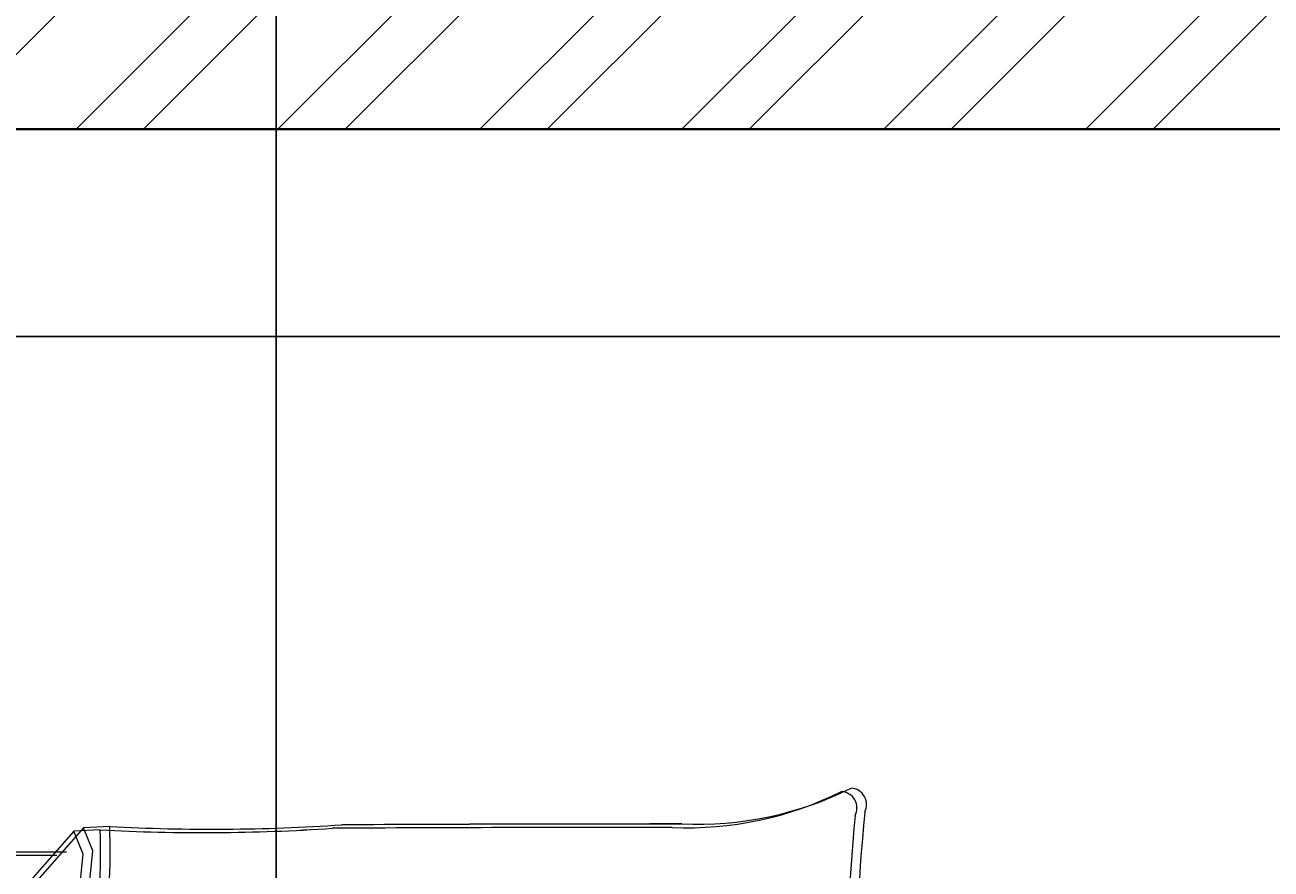
# Model space of a CAD drawing. Units: inches. Extents: x 1601 to 2297, y 1496 to 2631.
# Tile 12 of 57: x 1723 to 1806, y 1973 to 2029. Entities that reach past the tile are written whole.
import ezdxf

# ---------------------------------------------------------------- set-up
doc = ezdxf.new("R2010")
doc.units = ezdxf.units.IN
for name, color, linetype, lineweight in [('A-ANNO-DIMS', 2, 'Continuous', 18), ('A-FURN', 8, 'Continuous', 18), ('A-WALL', 7, 'Continuous', 40), ('A-WALL-PATT', 215, 'Continuous', 13)]:
    doc.layers.add(name, color=color, linetype=linetype, lineweight=lineweight)
doc.styles.get("Standard").update_dxf_attribs({"font": 'arial.ttf'})
doc.dimstyles.get("Standard").update_dxf_attribs({"dimtxt": 0.18, "dimasz": 0.18, "dimexe": 0.18, "dimexo": 0.0625, "dimgap": 0.09, "dimtad": 0, "dimtih": 1, "dimtoh": 1, "dimdec": 4, "dimzin": 0, "dimdsep": 46, "dimtxsty": 'Standard', "dimcen": 0.09, "dimadec": 0, "dimazin": 0, "dimtfac": 1, "dimtdec": 4, "dimtofl": 0, "dimtmove": 0, "dimatfit": 3, "dimfxl": 1, "dimtolj": 1, "dimtzin": 0, "dimarcsym": 0})

# ---------------------------------------------------------------- blocks, each defined once
blk = doc.blocks.new('BED-DOUBLE')
for p, q in [((27.746, 52.867), (24.495, 49.162)), ((27.746, 52.867), (24.495, 49.162)), ((27.746, 52.867), (24.495, 49.162)), ((27.746, 52.867), (24.495, 49.162)), ((28.385, 53.096), (25.135, 49.39)), ((28.385, 53.096), (25.135, 49.39)), ((28.385, 53.096), (25.135, 49.39)), ((28.385, 53.096), (25.135, 49.39)), ((29.49, 52.947), (27.746, 52.867, 3.871)), ((29.49, 52.947), (27.746, 52.867, 3.871)), ((29.49, 52.947), (27.746, 52.867, 3.871)), ((29.49, 52.947), (27.746, 52.867, 3.871)), ((28.365, 51.33), (27.746, 52.867)), ((28.365, 51.33), (27.746, 52.867)), ((28.365, 51.33), (27.746, 52.867)), ((28.365, 51.33), (27.746, 52.867)), ((30.13, 53.175), (28.385, 53.096, 3.871)), ((30.13, 53.175), (28.385, 53.096, 3.871)), ((30.13, 53.175), (28.385, 53.096, 3.871)), ((30.13, 53.175), (28.385, 53.096, 3.871)), ((29.004, 51.559), (28.385, 53.096)), ((29.004, 51.558), (28.385, 53.096)), ((29.004, 51.559), (28.385, 53.096)), ((29.004, 51.558), (28.385, 53.096)), ((28.695, 48.461), (29.004, 51.559)), ((28.695, 48.461), (29.004, 51.559)), ((28.695, 48.461), (29.004, 51.558)), ((28.695, 48.461), (29.004, 51.558)), ((0, 51.494), (0.639, 51.493)), ((0, 3.475), (0, 51.494)), ((0, 51.494), (0.639, 51.493)), ((0, 3.475), (0, 51.494)), ((0, 51.265), (26.61, 51.265)), ((0, 51.265), (26.61, 51.265)), ((0, 51.265), (26.61, 51.265)), ((0, 51.265), (26.61, 51.265)), ((0.639, 51.494), (27.249, 51.494)), ((0.639, 51.494), (27.249, 51.494)), ((0.639, 51.493), (27.249, 51.493)), ((0.639, 51.493), (27.249, 51.493)), ((1.533, 3.475), (1.533, 51.265)), ((1.533, 3.475), (1.533, 51.265)), ((1.533, 3.475), (1.533, 51.265)), ((1.533, 3.475), (1.533, 51.265)), ((2.173, 3.703), (2.173, 51.494)), ((2.173, 3.703), (2.173, 51.494)), ((2.173, 3.703), (2.173, 51.493)), ((2.173, 3.703), (2.173, 51.493)), ((17.212, 50.926), (14.073, 50.151)), ((17.212, 50.926), (14.073, 50.151)), ((17.212, 50.926), (14.073, 50.151)), ((17.212, 50.926), (14.073, 50.151)), ((16.808, 45.795), (17.212, 50.926)), ((16.808, 45.794), (17.212, 50.926)), ((16.808, 45.795), (17.212, 50.926)), ((16.808, 45.794), (17.212, 50.926)), ((28.055, 48.233), (28.365, 51.33)), ((28.055, 48.233), (28.365, 51.33)), ((28.055, 48.233), (28.365, 51.33)), ((28.055, 48.233), (28.365, 51.33)), ((2.557, 50.112), (2.46, 44.709)), ((2.557, 50.112), (2.46, 44.709)), ((2.557, 50.111), (2.46, 44.709)), ((2.557, 50.111), (2.46, 44.709)), ((2.557, 50.112), (5.768, 49.733)), ((2.557, 50.112), (5.768, 49.733)), ((2.557, 50.111), (5.768, 49.733)), ((2.557, 50.111), (5.768, 49.733)), ((3.196, 50.34), (3.099, 44.938)), ((3.196, 50.34), (3.099, 44.938)), ((3.196, 50.34), (3.099, 44.938)), ((3.196, 50.34), (3.099, 44.938)), ((3.196, 50.34), (6.407, 49.961)), ((3.196, 50.34), (6.407, 49.961)), ((3.196, 50.34), (6.407, 49.961)), ((3.196, 50.34), (6.407, 49.961)), ((5.768, 49.733), (8.338, 50.328)), ((5.768, 49.733), (8.338, 50.328)), ((5.768, 49.733), (8.338, 50.328)), ((5.768, 49.733), (8.338, 50.328)), ((6.407, 49.961), (8.977, 50.557)), ((6.407, 49.961), (8.977, 50.557)), ((6.407, 49.961), (8.977, 50.556)), ((6.407, 49.961), (8.977, 50.556)), ((11.829, 50.112), (8.257, 49.309)), ((11.829, 50.112), (8.257, 49.309)), ((11.829, 50.112), (8.257, 49.309)), ((11.829, 50.112), (8.257, 49.309)), ((8.338, 50.328), (9.384, 49.814)), ((8.338, 50.328), (9.384, 49.814)), ((8.338, 50.328), (9.384, 49.814)), ((8.338, 50.328), (9.384, 49.814)), ((12.468, 50.34), (8.896, 49.538)), ((12.468, 50.34), (8.896, 49.537)), ((12.468, 50.34), (8.896, 49.538)), ((12.468, 50.34), (8.896, 49.537)), ((8.977, 50.557), (10.024, 50.043)), ((8.977, 50.557), (10.024, 50.043)), ((8.977, 50.556), (10.024, 50.042)), ((8.977, 50.556), (10.024, 50.042)), ((13.434, 49.923), (11.829, 50.112)), ((13.434, 49.922), (11.829, 50.112)), ((13.434, 49.923), (11.829, 50.112)), ((13.434, 49.922), (11.829, 50.112)), ((14.073, 50.151), (12.468, 50.34)), ((14.073, 50.151), (12.468, 50.34)), ((14.073, 50.151), (12.468, 50.34)), ((14.073, 50.151), (12.468, 50.34)), ((16.573, 50.698), (13.434, 49.923)), ((16.573, 50.698), (13.434, 49.922)), ((16.573, 50.698), (13.434, 49.923)), ((16.573, 50.698), (13.434, 49.922)), ((16.169, 45.566), (16.573, 50.698)), ((16.169, 45.566), (16.573, 50.698)), ((16.169, 45.566), (16.573, 50.698)), ((16.169, 45.566), (16.573, 50.698)), ((8.257, 49.309), (5.578, 48.128)), ((8.257, 49.309), (5.578, 48.128)), ((8.257, 49.309), (5.578, 48.128)), ((8.257, 49.309), (5.578, 48.128)), ((8.896, 49.538), (6.218, 48.356)), ((8.896, 49.538), (6.218, 48.356)), ((8.896, 49.537), (6.218, 48.356)), ((8.896, 49.537), (6.218, 48.356)), ((24.495, 49.162), (22.329, 46.219)), ((24.495, 49.162), (22.329, 46.219)), ((24.495, 49.162), (22.329, 46.219)), ((24.495, 49.162), (22.329, 46.219)), ((25.135, 49.39), (22.968, 46.448)), ((25.135, 49.39), (22.968, 46.448)), ((25.135, 49.39), (22.968, 46.448)), ((25.135, 49.39), (22.968, 46.448)), ((28.365, 44.361), (28.055, 48.233)), ((28.365, 44.361), (28.055, 48.233)), ((28.365, 44.361), (28.055, 48.233)), ((28.365, 44.361), (28.055, 48.233)), ((29.004, 44.589), (28.695, 48.461)), ((29.004, 44.589), (28.695, 48.461)), ((29.004, 44.589), (28.695, 48.461)), ((29.004, 44.589), (28.695, 48.461)), ((3.099, 44.938), (3.181, 45.941)), ((3.099, 44.938), (3.181, 45.941)), ((3.099, 44.938), (3.181, 45.94)), ((3.099, 44.938), (3.181, 45.94)), ((3.181, 45.941), (3.709, 42.143)), ((3.181, 45.941), (3.709, 42.143)), ((3.181, 45.94), (3.709, 42.142)), ((3.181, 45.94), (3.709, 42.142)), ((17.365, 43.834), (16.808, 45.795)), ((17.365, 43.834), (16.808, 45.795)), ((17.365, 43.834), (16.808, 45.794)), ((17.365, 43.834), (16.808, 45.794)), ((22.329, 46.219), (20.316, 40.644)), ((22.329, 46.219), (20.316, 40.644)), ((22.329, 46.219), (20.317, 40.644)), ((22.329, 46.219), (20.317, 40.644)), ((22.968, 46.448), (20.956, 40.872)), ((22.968, 46.448), (20.956, 40.872)), ((22.968, 46.448), (20.956, 40.872)), ((22.968, 46.448), (20.956, 40.872)), ((2.46, 44.709), (2.542, 45.712)), ((2.46, 44.709), (2.542, 45.712)), ((2.46, 44.709), (2.542, 45.712)), ((2.46, 44.709), (2.542, 45.712)), ((2.542, 45.712), (3.069, 41.914)), ((2.542, 45.712), (3.069, 41.914)), ((2.542, 45.712), (3.069, 41.914)), ((2.542, 45.712), (3.069, 41.914)), ((16.726, 43.606), (16.169, 45.566)), ((16.726, 43.606), (16.169, 45.566)), ((16.726, 43.606), (16.169, 45.566)), ((16.726, 43.606), (16.169, 45.566)), ((28.829, 40.954), (28.365, 44.361)), ((28.829, 40.953), (28.365, 44.361)), ((28.829, 40.954), (28.365, 44.361)), ((28.829, 40.953), (28.365, 44.361)), ((29.468, 41.182), (29.004, 44.589)), ((29.469, 41.182), (29.004, 44.589)), ((29.468, 41.182), (29.004, 44.589)), ((29.469, 41.182), (29.004, 44.589)), ((16.295, 36.596), (16.726, 43.606)), ((16.295, 36.596), (16.726, 43.606)), ((16.295, 36.596), (16.726, 43.606)), ((16.295, 36.596), (16.726, 43.606)), ((16.934, 36.824), (17.365, 43.834)), ((16.934, 36.824), (17.365, 43.834)), ((16.934, 36.824), (17.365, 43.834)), ((16.934, 36.824), (17.365, 43.834)), ((3.069, 41.914), (4.422, 36.495)), ((3.069, 41.914), (4.422, 36.495)), ((3.069, 41.914), (4.422, 36.495)), ((3.069, 41.914), (4.422, 36.495)), ((3.709, 42.143), (5.061, 36.723)), ((3.709, 42.143), (5.061, 36.723)), ((3.709, 42.142), (5.061, 36.723)), ((3.709, 42.142), (5.061, 36.723)), ((20.956, 40.872), (18.022, 32.534)), ((20.956, 40.872), (18.022, 32.534)), ((20.956, 40.872), (18.022, 32.534)), ((20.956, 40.872), (18.022, 32.534)), ((29.758, 38.94), (28.829, 40.954)), ((29.758, 38.94), (28.829, 40.954)), ((29.758, 38.94), (28.829, 40.953)), ((29.758, 38.94), (28.829, 40.953)), ((30.397, 39.169), (29.468, 41.182)), ((30.397, 39.169), (29.468, 41.182)), ((30.397, 39.168), (29.469, 41.182)), ((30.397, 39.168), (29.469, 41.182)), ((20.316, 40.644), (17.383, 32.306)), ((20.317, 40.644), (17.383, 32.306)), ((20.316, 40.644), (17.383, 32.306)), ((20.317, 40.644), (17.383, 32.306)), ((79.884, 15.292), (79.884, 39.905)), ((79.884, 15.291), (79.884, 39.905)), ((79.884, 15.292), (79.884, 39.905)), ((79.884, 15.291), (79.884, 39.905)), ((3.673, 39.2), (3.078, 37.135)), ((3.673, 39.2), (3.078, 37.135)), ((3.673, 39.2), (3.078, 37.135)), ((3.673, 39.2), (3.078, 37.135)), ((4.313, 39.428), (3.717, 37.363)), ((4.313, 39.428), (3.717, 37.363)), ((4.313, 39.428), (3.718, 37.363)), ((4.313, 39.428), (3.718, 37.363)), ((31.016, 36.691), (30.397, 39.169)), ((31.016, 36.691), (30.397, 39.169)), ((31.016, 36.691), (30.397, 39.168)), ((31.016, 36.691), (30.397, 39.168)), ((79.245, 15.063), (79.245, 39.677)), ((79.245, 15.063), (79.245, 39.677)), ((79.245, 15.063), (79.245, 39.677)), ((79.245, 15.063), (79.245, 39.677)), ((30.377, 36.462), (29.758, 38.94)), ((30.377, 36.462), (29.758, 38.94)), ((30.377, 36.462), (29.758, 38.94)), ((30.377, 36.462), (29.758, 38.94)), ((3.078, 37.135), (2.537, 34.204)), ((3.078, 37.135), (2.537, 34.204)), ((3.078, 37.135), (2.537, 34.204)), ((3.078, 37.135), (2.537, 34.204)), ((3.717, 37.363), (3.176, 34.433)), ((3.718, 37.363), (3.176, 34.433)), ((3.717, 37.363), (3.176, 34.433)), ((3.718, 37.363), (3.176, 34.433)), ((15.628, 32.564), (16.295, 36.596)), ((15.628, 32.564), (16.295, 36.596)), ((15.628, 32.564), (16.295, 36.596)), ((15.628, 32.564), (16.295, 36.596)), ((16.268, 32.792), (16.934, 36.824)), ((16.268, 32.792), (16.934, 36.824)), ((16.268, 32.792), (16.934, 36.824)), ((16.268, 32.792), (16.934, 36.824)), ((29.004, 36.381), (31.016, 36.691)), ((29.004, 36.381), (31.016, 36.691)), ((29.004, 36.381), (31.016, 36.691)), ((29.004, 36.381), (31.016, 36.691)), ((23.876, 34.449), (28.365, 36.153)), ((23.876, 34.449), (28.365, 36.153)), ((23.876, 34.449), (28.365, 36.152)), ((23.876, 34.449), (28.365, 36.152)), ((24.516, 34.677), (29.004, 36.381)), ((24.516, 34.677), (29.004, 36.381)), ((24.516, 34.677), (29.004, 36.381)), ((24.516, 34.677), (29.004, 36.381)), ((28.365, 36.153), (30.377, 36.462)), ((28.365, 36.152), (30.377, 36.462)), ((28.365, 36.153), (30.377, 36.462)), ((28.365, 36.152), (30.377, 36.462)), ((2.537, 34.204), (2.557, 33.883)), ((2.537, 34.204), (2.557, 33.883)), ((2.537, 34.204), (2.557, 33.883)), ((2.537, 34.204), (2.557, 33.883)), ((3.176, 34.433), (3.196, 34.112)), ((3.176, 34.433), (3.196, 34.112)), ((3.176, 34.433), (3.196, 34.112)), ((3.176, 34.433), (3.196, 34.112)), ((3.196, 34.112), (3.618, 29.684)), ((3.196, 34.112), (3.618, 29.684)), ((3.196, 34.112), (3.618, 29.684)), ((3.196, 34.112), (3.618, 29.684)), ((17.383, 30.259), (23.876, 34.449)), ((17.383, 30.259), (23.876, 34.449)), ((17.383, 30.259), (23.876, 34.449)), ((17.383, 30.259), (23.876, 34.449)), ((18.022, 30.487), (24.516, 34.677)), ((18.022, 30.487), (24.516, 34.677)), ((18.022, 30.487), (24.516, 34.677)), ((18.022, 30.487), (24.516, 34.677)), ((2.557, 33.883), (2.979, 29.456)), ((2.557, 33.883), (2.979, 29.455)), ((2.557, 33.883), (2.979, 29.456)), ((2.557, 33.883), (2.979, 29.455)), ((16.739, 30.75), (15.454, 33.821)), ((16.739, 30.75), (15.454, 33.821)), ((16.739, 30.75), (15.454, 33.82)), ((16.739, 30.75), (15.454, 33.82)), ((17.379, 30.978), (16.094, 34.049)), ((17.379, 30.978), (16.094, 34.049)), ((17.379, 30.978), (16.094, 34.049)), ((17.379, 30.978), (16.094, 34.049)), ((17.532, 28.526), (17.379, 30.978)), ((17.532, 28.525), (17.379, 30.978)), ((17.532, 28.526), (17.379, 30.978)), ((17.532, 28.525), (17.379, 30.978)), ((16.893, 28.297), (16.739, 30.75)), ((16.893, 28.297), (16.739, 30.75)), ((16.893, 28.297), (16.739, 30.75)), ((16.893, 28.297), (16.739, 30.75)), ((2.979, 29.456), (2.492, 27.977)), ((2.979, 29.456), (2.492, 27.977)), ((2.979, 29.455), (2.492, 27.976)), ((2.979, 29.455), (2.492, 27.976)), ((3.618, 29.684), (3.131, 28.205)), ((3.618, 29.684), (3.131, 28.205)), ((3.618, 29.684), (3.131, 28.205)), ((3.618, 29.684), (3.131, 28.205)), ((13.016, 27.664), (14.856, 28.359)), ((13.016, 27.664), (14.856, 28.359)), ((13.016, 27.664), (14.856, 28.358)), ((13.016, 27.664), (14.856, 28.358)), ((14.216, 28.13), (16.893, 28.297)), ((14.216, 28.13), (16.893, 28.297)), ((14.217, 28.13), (16.893, 28.297)), ((14.217, 28.13), (16.893, 28.297)), ((14.856, 28.359), (17.532, 28.526)), ((14.856, 28.359), (17.532, 28.526)), ((14.856, 28.358), (17.532, 28.525)), ((14.856, 28.358), (17.532, 28.525)), ((2.492, 27.977), (7.867, 27.733)), ((2.492, 27.977), (7.867, 27.733)), ((2.492, 27.976), (7.867, 27.733)), ((2.492, 27.976), (7.867, 27.733)), ((3.131, 28.205), (8.506, 27.962)), ((3.131, 28.205), (8.506, 27.961)), ((3.131, 28.205), (8.506, 27.962)), ((3.131, 28.205), (8.506, 27.961)), ((7.867, 27.733), (11.078, 27.355)), ((7.867, 27.733), (11.078, 27.354)), ((7.867, 27.733), (11.078, 27.355)), ((7.867, 27.733), (11.078, 27.354)), ((8.506, 27.962), (11.717, 27.583)), ((8.506, 27.962), (11.717, 27.583)), ((8.506, 27.961), (11.717, 27.583)), ((8.506, 27.961), (11.717, 27.583)), ((11.078, 27.355), (12.377, 27.436)), ((11.078, 27.354), (12.377, 27.436)), ((11.078, 27.355), (12.377, 27.436)), ((11.078, 27.354), (12.377, 27.436)), ((11.717, 27.583), (13.016, 27.664)), ((11.717, 27.583), (13.016, 27.664)), ((11.717, 27.583), (13.016, 27.664)), ((11.717, 27.583), (13.016, 27.664)), ((12.377, 27.436), (14.216, 28.13)), ((12.377, 27.436), (14.217, 28.13)), ((12.377, 27.436), (14.216, 28.13)), ((12.377, 27.436), (14.217, 28.13)), ((2.509, 26.211), (7.859, 26.789)), ((2.509, 26.21), (7.859, 26.789)), ((2.509, 26.211), (7.859, 26.789)), ((2.509, 26.21), (7.859, 26.789)), ((7.22, 26.561), (10.401, 27.139)), ((7.22, 26.56), (10.401, 27.139)), ((7.22, 26.561), (10.401, 27.139)), ((7.22, 26.56), (10.401, 27.139)), ((7.859, 26.789), (11.04, 27.367)), ((7.859, 26.789), (11.04, 27.367)), ((7.859, 26.789), (11.04, 27.367)), ((7.859, 26.789), (11.04, 27.367)), ((10.401, 27.139), (11.702, 27.139)), ((10.401, 27.139), (11.702, 27.139)), ((10.401, 27.139), (11.702, 27.139)), ((10.401, 27.139), (11.702, 27.139)), ((11.04, 27.367), (12.341, 27.367)), ((11.04, 27.367), (12.341, 27.367)), ((11.04, 27.367), (12.341, 27.367)), ((11.04, 27.367), (12.341, 27.367)), ((11.702, 27.139), (13.582, 26.561)), ((11.702, 27.139), (13.582, 26.56)), ((11.702, 27.139), (13.582, 26.561)), ((11.702, 27.139), (13.582, 26.56)), ((12.341, 27.367), (14.221, 26.789)), ((12.341, 27.367), (14.221, 26.789)), ((12.341, 27.367), (14.221, 26.789)), ((12.341, 27.367), (14.221, 26.789)), ((14.221, 26.789), (16.902, 26.789)), ((14.221, 26.789), (16.902, 26.789)), ((14.221, 26.789), (16.902, 26.789)), ((14.221, 26.789), (16.902, 26.789)), ((16.902, 26.789), (16.902, 24.332)), ((16.902, 26.789), (16.902, 24.331)), ((16.902, 26.789), (16.902, 24.332)), ((16.902, 26.789), (16.902, 24.331)), ((1.87, 25.982), (7.22, 26.561)), ((1.87, 25.982), (7.22, 26.561)), ((1.87, 25.982), (7.22, 26.56)), ((1.87, 25.982), (7.22, 26.56)), ((2.448, 24.537), (1.87, 25.982)), ((2.448, 24.537), (1.87, 25.982)), ((2.448, 24.537), (1.87, 25.982)), ((2.448, 24.537), (1.87, 25.982)), ((3.088, 24.765), (2.509, 26.211)), ((3.088, 24.765), (2.509, 26.211)), ((3.088, 24.765), (2.509, 26.21)), ((3.088, 24.765), (2.509, 26.21)), ((13.582, 26.561), (16.263, 26.561)), ((13.582, 26.561), (16.263, 26.561)), ((13.582, 26.56), (16.263, 26.56)), ((13.582, 26.56), (16.263, 26.56)), ((16.263, 26.561), (16.263, 24.103)), ((16.263, 26.561), (16.263, 24.103)), ((16.263, 26.56), (16.263, 24.103)), ((16.263, 26.56), (16.263, 24.103)), ((2.304, 20.091), (2.448, 24.537)), ((2.304, 20.091), (2.448, 24.537)), ((2.304, 20.091), (2.448, 24.537)), ((2.304, 20.091), (2.448, 24.537)), ((2.943, 20.32), (3.088, 24.765)), ((2.943, 20.319), (3.088, 24.765)), ((2.943, 20.32), (3.088, 24.765)), ((2.943, 20.319), (3.088, 24.765)), ((16.263, 24.103), (15.172, 20.959)), ((16.263, 24.103), (15.172, 20.959)), ((16.902, 24.332), (15.811, 21.187)), ((16.902, 24.332), (15.811, 21.187)), ((16.902, 24.331), (15.811, 21.187)), ((16.902, 24.331), (15.811, 21.187)), ((16.169, 19.384), (16.573, 24.516)), ((16.169, 19.384), (16.573, 24.516)), ((16.169, 19.383), (16.573, 24.515)), ((16.169, 19.383), (16.573, 24.515)), ((16.808, 19.612), (17.212, 24.744)), ((16.808, 19.612), (17.212, 24.744)), ((16.808, 19.612), (17.212, 24.744)), ((16.808, 19.612), (17.212, 24.744)), ((16.263, 24.103), (15.172, 20.958)), ((16.263, 24.103), (15.172, 20.958)), ((2.304, 19.77), (2.304, 20.091)), ((2.304, 19.769), (2.304, 20.091)), ((2.304, 19.77), (2.304, 20.091)), ((2.304, 19.769), (2.304, 20.091)), ((2.943, 19.998), (2.943, 20.32)), ((2.943, 19.998), (2.943, 20.32)), ((2.943, 19.998), (2.943, 20.319)), ((2.943, 19.998), (2.943, 20.319)), ((3.666, 17.107), (2.943, 19.998)), ((3.666, 17.107), (2.943, 19.998)), ((3.666, 17.107), (2.943, 19.998)), ((3.666, 17.107), (2.943, 19.998)), ((3.027, 16.878), (2.304, 19.77)), ((3.027, 16.878), (2.304, 19.77)), ((3.027, 16.878), (2.304, 19.769)), ((3.027, 16.878), (2.304, 19.769)), ((16.726, 17.423), (16.169, 19.384)), ((16.726, 17.423), (16.169, 19.384)), ((16.726, 17.423), (16.169, 19.383)), ((16.726, 17.423), (16.169, 19.383)), ((17.365, 17.652), (16.808, 19.612)), ((17.365, 17.651), (16.808, 19.612)), ((17.365, 17.652), (16.808, 19.612)), ((17.365, 17.651), (16.808, 19.612)), ((3.316, 12.108), (4.328, 17.601)), ((3.316, 12.108), (4.328, 17.601)), ((3.316, 12.108), (4.328, 17.601)), ((3.316, 12.108), (4.328, 17.601)), ((3.955, 12.336), (4.967, 17.83)), ((3.955, 12.336), (4.967, 17.83)), ((3.955, 12.336), (4.967, 17.829)), ((3.955, 12.336), (4.967, 17.829)), ((16.934, 10.642), (17.365, 17.652)), ((16.934, 10.642), (17.365, 17.652)), ((16.934, 10.642), (17.365, 17.651)), ((16.934, 10.642), (17.365, 17.651)), ((3.75, 14.855), (3.027, 16.878)), ((3.75, 14.854), (3.027, 16.878)), ((3.75, 14.855), (3.027, 16.878)), ((3.75, 14.854), (3.027, 16.878)), ((4.389, 15.083), (3.666, 17.107)), ((4.389, 15.083), (3.666, 17.107)), ((4.389, 15.083), (3.666, 17.107)), ((4.389, 15.083), (3.666, 17.107)), ((16.295, 10.413), (16.726, 17.423)), ((16.295, 10.413), (16.726, 17.423)), ((16.295, 10.413), (16.726, 17.423)), ((16.295, 10.413), (16.726, 17.423)), ((3.027, 8.285), (3.316, 12.108)), ((3.027, 8.284), (3.316, 12.108)), ((3.027, 8.285), (3.316, 12.108)), ((3.027, 8.284), (3.316, 12.108)), ((3.666, 8.513), (3.955, 12.336)), ((3.666, 8.513), (3.955, 12.336)), ((3.666, 8.513), (3.955, 12.336)), ((3.666, 8.513), (3.955, 12.336)), ((15.628, 6.382), (16.295, 10.413)), ((15.628, 6.381), (16.295, 10.413)), ((15.628, 6.382), (16.295, 10.413)), ((15.628, 6.381), (16.295, 10.413)), ((16.268, 6.61), (16.934, 10.642)), ((16.268, 6.61), (16.934, 10.642)), ((16.268, 6.61), (16.934, 10.642)), ((16.268, 6.61), (16.934, 10.642)), ((16.295, 10.413), (16.618, 9.28)), ((16.295, 10.413), (16.618, 9.28)), ((16.295, 10.413), (16.618, 9.28)), ((16.295, 10.413), (16.618, 9.28)), ((16.934, 10.642), (17.257, 9.509)), ((16.934, 10.642), (17.257, 9.508)), ((16.934, 10.642), (17.257, 9.509)), ((16.934, 10.642), (17.257, 9.508)), ((16.618, 9.28), (17.341, 4.184)), ((16.618, 9.28), (17.341, 4.183)), ((16.618, 9.28), (17.341, 4.184)), ((16.618, 9.28), (17.341, 4.183)), ((17.257, 9.509), (17.98, 4.412)), ((17.257, 9.509), (17.98, 4.412)), ((17.257, 9.508), (17.98, 4.412)), ((17.257, 9.508), (17.98, 4.412)), ((3.648, 8.408), (3.666, 8.513)), ((3.648, 8.407), (3.666, 8.513)), ((3.648, 8.408), (3.666, 8.513)), ((3.648, 8.407), (3.666, 8.513)), ((3.977, 4.127), (3.648, 8.408)), ((3.977, 4.127), (3.648, 8.408)), ((3.977, 4.127), (3.648, 8.407)), ((3.977, 4.127), (3.648, 8.407)), ((3.009, 8.179), (3.027, 8.285)), ((3.009, 8.179), (3.027, 8.285)), ((3.009, 8.179), (3.027, 8.284)), ((3.009, 8.179), (3.027, 8.284)), ((3.338, 3.898), (3.009, 8.179)), ((3.338, 3.898), (3.009, 8.179)), ((3.338, 3.898), (3.009, 8.179)), ((3.338, 3.898), (3.009, 8.179)), ((8.955, 5.051), (6.208, 6.063)), ((8.955, 5.051), (6.208, 6.063)), ((8.955, 5.051), (6.208, 6.063)), ((8.955, 5.051), (6.208, 6.063)), ((9.594, 5.279), (6.847, 6.291)), ((9.594, 5.279), (6.847, 6.291)), ((9.594, 5.279), (6.847, 6.291)), ((9.594, 5.279), (6.847, 6.291)), ((12.57, 4.473), (8.955, 5.051)), ((12.57, 4.472), (8.955, 5.051)), ((12.57, 4.473), (8.955, 5.051)), ((12.57, 4.472), (8.955, 5.051)), ((13.209, 4.701), (9.594, 5.279)), ((13.209, 4.701), (9.594, 5.279)), ((13.209, 4.701), (9.594, 5.279)), ((13.209, 4.701), (9.594, 5.279)), ((14.799, 4.99), (13.209, 4.701)), ((14.799, 4.99), (13.209, 4.701)), ((14.799, 4.99), (13.209, 4.701)), ((14.799, 4.99), (13.209, 4.701)), ((17.98, 4.412), (14.799, 4.99)), ((17.98, 4.412), (14.799, 4.99)), ((17.98, 4.412), (14.799, 4.99)), ((17.98, 4.412), (14.799, 4.99)), ((3.316, 3.894), (6.497, 4.473)), ((3.316, 3.894), (6.497, 4.473)), ((3.316, 3.894), (6.497, 4.472)), ((3.316, 3.894), (6.497, 4.472)), ((3.955, 4.123), (7.136, 4.701)), ((3.955, 4.123), (7.136, 4.701)), ((3.955, 4.123), (7.136, 4.701)), ((3.955, 4.123), (7.136, 4.701)), ((6.497, 4.473), (9.099, 4.039)), ((6.497, 4.473), (9.099, 4.039)), ((6.497, 4.472), (9.099, 4.039)), ((6.497, 4.472), (9.099, 4.039)), ((7.136, 4.701), (9.739, 4.267)), ((7.136, 4.701), (9.739, 4.267)), ((7.136, 4.701), (9.739, 4.267)), ((7.136, 4.701), (9.739, 4.267)), ((9.099, 4.039), (10.112, 4.617)), ((9.099, 4.039), (10.112, 4.617)), ((9.099, 4.039), (10.112, 4.617)), ((9.099, 4.039), (10.112, 4.617)), ((9.739, 4.267), (10.751, 4.846)), ((9.739, 4.267), (10.751, 4.846)), ((9.739, 4.267), (10.751, 4.845)), ((9.739, 4.267), (10.751, 4.845)), ((14.16, 4.762), (12.57, 4.473)), ((14.16, 4.762), (12.57, 4.472)), ((14.16, 4.762), (12.57, 4.473)), ((14.16, 4.762), (12.57, 4.472)), ((17.341, 4.184), (14.16, 4.762)), ((17.341, 4.183), (14.16, 4.762)), ((17.341, 4.184), (14.16, 4.762)), ((17.341, 4.183), (14.16, 4.762)), ((18.11, 3.475), (0, 3.475)), ((18.11, 3.475), (0, 3.475)), ((18.11, 3.475), (0, 3.475)), ((18.11, 3.475), (0, 3.475)), ((18.75, 3.703), (0.639, 3.703)), ((18.75, 3.703), (0.639, 3.703)), ((18.75, 3.703), (0.639, 3.703)), ((18.75, 3.703), (0.639, 3.703))]:
    blk.add_line(p, q)
for centre, radius, start, end in [((69.306, 76.385), 23.065, 267.47136, 296.46809), ((69.306, 76.385), 23.065, 267.47136, 296.46809), ((69.306, 76.385), 23.065, 267.47136, 296.46809), ((69.306, 76.385), 23.065, 267.47136, 296.46809), ((79.509, 54.638), 1.102, 332.65876, 86.02002), ((79.509, 54.638), 1.102, 332.65876, 86.02002), ((79.509, 54.638), 1.102, 332.65876, 86.02002), ((79.509, 54.638), 1.102, 332.65876, 86.02002), ((68.666, 76.157), 23.065, 267.47136, 296.46809), ((68.666, 76.157), 23.065, 267.47136, 296.46809), ((68.666, 76.157), 23.065, 267.47136, 296.46809), ((68.666, 76.157), 23.065, 267.47136, 296.46809), ((78.87, 54.41), 1.102, 332.65876, 86.02002), ((78.87, 54.409), 1.102, 332.65876, 86.02002), ((78.87, 54.41), 1.102, 332.65876, 86.02002), ((78.87, 54.409), 1.102, 332.65876, 86.02002), ((212.916, 41.38), 133.04, 174.4998, 180.63509), ((212.916, 41.38), 133.04, 174.4998, 180.63509), ((212.916, 41.38), 133.04, 174.4998, 180.63509), ((212.916, 41.38), 133.04, 174.4998, 180.63509), ((36.954, 182.494), 129.499, 266.97912, 273.83645), ((36.954, 182.494), 129.499, 266.97912, 273.83645), ((36.954, 182.494), 129.499, 266.97912, 273.83645), ((36.954, 182.494), 129.499, 266.97912, 273.83645), ((68.461, -4508.515), 4561.858, 90.002168, 90.286887), ((68.461, -4508.515), 4561.858, 90.002168, 90.286887), ((68.461, -4508.516), 4561.858, 90.002168, 90.286887), ((68.461, -4508.516), 4561.858, 90.002168, 90.286887), ((212.276, 41.152), 133.04, 174.4998, 180.63509), ((212.277, 41.151), 133.04, 174.4998, 180.63509), ((212.276, 41.152), 133.04, 174.4998, 180.63509), ((212.277, 41.151), 133.04, 174.4998, 180.63509), ((-6.656, 51.327), 36.183, 349.87628, 2.56571), ((-6.656, 51.327), 36.183, 349.87628, 2.56571), ((-6.656, 51.327), 36.183, 349.87628, 2.56571), ((-6.656, 51.327), 36.183, 349.87628, 2.56571), ((36.315, 182.266), 129.499, 266.97912, 273.83645), ((36.315, 182.265), 129.499, 266.97912, 273.83645), ((36.315, 182.266), 129.499, 266.97912, 273.83645), ((36.315, 182.265), 129.499, 266.97912, 273.83645), ((-6.017, 51.555), 36.183, 349.87628, 2.56571), ((-6.017, 51.555), 36.183, 349.87628, 2.56571), ((-6.017, 51.555), 36.183, 349.87628, 2.56571), ((-6.017, 51.555), 36.183, 349.87628, 2.56571), ((67.821, -4508.744), 4561.858, 90.002168, 90.286887), ((67.821, -4508.744), 4561.858, 90.002168, 90.286887), ((67.821, -4508.744), 4561.858, 90.002168, 90.286887), ((67.821, -4508.744), 4561.858, 90.002168, 90.286887), ((35.066, 43.743), 6.224, 168.6608, 203.73842), ((35.066, 43.743), 6.224, 168.6608, 203.73842), ((35.066, 43.743), 6.224, 168.6608, 203.73842), ((35.066, 43.743), 6.224, 168.6608, 203.73842), ((35.705, 43.972), 6.224, 168.6608, 203.73842), ((35.705, 43.971), 6.224, 168.6608, 203.73842), ((35.705, 43.972), 6.224, 168.6608, 203.73842), ((35.705, 43.971), 6.224, 168.6608, 203.73842), ((1.482, 31.154), 29.654, 10.66171, 19.88058), ((1.482, 31.154), 29.654, 10.66171, 19.88058), ((1.482, 31.153), 29.654, 10.66171, 19.88058), ((1.482, 31.153), 29.654, 10.66171, 19.88058), ((2.121, 31.382), 29.654, 10.66171, 19.88058), ((2.121, 31.382), 29.654, 10.66171, 19.88058), ((2.121, 31.382), 29.654, 10.66171, 19.88058), ((2.121, 31.382), 29.654, 10.66171, 19.88058), ((30.439, 36.636), 0.185, 250.24637, 1.13765), ((30.439, 36.636), 0.185, 250.24637, 1.13765), ((30.439, 36.636), 0.185, 250.24637, 1.13765), ((30.439, 36.636), 0.185, 250.24637, 1.13765), ((31.079, 36.864), 0.185, 250.24637, 1.13765), ((31.079, 36.864), 0.185, 250.24637, 1.13765), ((31.079, 36.864), 0.185, 250.24637, 1.13765), ((31.079, 36.864), 0.185, 250.24637, 1.13765), ((156.316, 17.756), 129.02, 171.78449, 186.90062), ((156.316, 17.755), 129.02, 171.78449, 186.90062), ((156.316, 17.756), 129.02, 171.78449, 186.90062), ((156.316, 17.755), 129.02, 171.78449, 186.90062), ((156.955, 17.984), 129.02, 171.78449, 186.90062), ((156.955, 17.984), 129.02, 171.78449, 186.90062), ((156.955, 17.984), 129.02, 171.78449, 186.90062), ((156.955, 17.984), 129.02, 171.78449, 186.90062), ((182.052, 21.359), 164.969, 176.08655, 186.78213), ((182.052, 21.359), 164.969, 176.08655, 186.78213), ((182.052, 21.358), 164.969, 176.08655, 186.78213), ((182.052, 21.358), 164.969, 176.08655, 186.78213), ((182.692, 21.587), 164.969, 176.08655, 186.78213), ((182.692, 21.587), 164.969, 176.08655, 186.78213), ((182.692, 21.587), 164.969, 176.08655, 186.78213), ((182.692, 21.587), 164.969, 176.08655, 186.78213), ((-23.712, -17.222), 106.459, 13.38322, 17.70533), ((-23.712, -17.222), 106.459, 13.38322, 17.70533), ((-23.712, -17.222), 106.459, 13.38322, 17.70533), ((-23.712, -17.222), 106.459, 13.38322, 17.70533), ((-23.073, -16.994), 106.459, 13.38322, 17.70533), ((-23.073, -16.994), 106.459, 13.38322, 17.70533), ((-23.073, -16.994), 106.459, 13.38322, 17.70533), ((-23.073, -16.994), 106.459, 13.38322, 17.70533), ((200.837, 21.427), 121.759, 182.99578, 189.40907), ((200.837, 21.426), 121.759, 182.99578, 189.40907), ((200.837, 21.427), 121.759, 182.99578, 189.40907), ((200.837, 21.426), 121.759, 182.99578, 189.40907), ((201.476, 21.655), 121.759, 182.99578, 189.40907), ((201.476, 21.655), 121.759, 182.99578, 189.40907), ((201.476, 21.655), 121.759, 182.99578, 189.40907), ((201.476, 21.655), 121.759, 182.99578, 189.40907), ((31.174, -167.308), 170.11, 88.4762, 91.00819), ((31.174, -167.308), 170.11, 88.4762, 91.00819), ((31.174, -167.308), 170.11, 88.4762, 91.00819), ((31.174, -167.308), 170.11, 88.4762, 91.00819), ((31.813, -167.079), 170.11, 88.4762, 91.00819), ((31.813, -167.08), 170.11, 88.4762, 91.00819), ((31.813, -167.079), 170.11, 88.4762, 91.00819), ((31.813, -167.08), 170.11, 88.4762, 91.00819), ((50.614, 484.822), 482.31, 268.22771, 271.71854), ((50.614, 484.822), 482.31, 268.22771, 271.71854), ((50.614, 484.822), 482.31, 268.22771, 271.71854), ((50.614, 484.822), 482.31, 268.22771, 271.71854), ((51.253, 485.051), 482.31, 268.22771, 271.71854), ((51.253, 485.05), 482.31, 268.22771, 271.71854), ((51.253, 485.051), 482.31, 268.22771, 271.71854), ((51.253, 485.05), 482.31, 268.22771, 271.71854), ((64.515, -26.9), 29.634, 76.06484, 88.91125), ((64.515, -26.9), 29.634, 76.06484, 88.91125), ((64.515, -26.9), 29.634, 76.06484, 88.91125), ((64.515, -26.9), 29.634, 76.06484, 88.91125), ((65.154, -26.671), 29.634, 76.06484, 88.91125), ((65.154, -26.672), 29.634, 76.06484, 88.91125), ((65.154, -26.671), 29.634, 76.06484, 88.91125), ((65.154, -26.672), 29.634, 76.06484, 88.91125), ((20.096, 85.162), 83.306, 268.72178, 275.60397), ((20.096, 85.161), 83.306, 268.72178, 275.60397), ((20.096, 85.162), 83.306, 268.72178, 275.60397), ((20.096, 85.161), 83.306, 268.72178, 275.60397), ((20.735, 85.39), 83.306, 268.72178, 275.60397), ((20.735, 85.39), 83.306, 268.72178, 275.60397), ((20.736, 85.39), 83.306, 268.72178, 275.60397), ((20.736, 85.39), 83.306, 268.72178, 275.60397), ((70.276, -21.66), 23.562, 67.97508, 86.652), ((70.276, -21.66), 23.562, 67.97508, 86.652), ((70.276, -21.66), 23.562, 67.97508, 86.652), ((70.276, -21.66), 23.562, 67.97508, 86.652), ((70.915, -21.431), 23.562, 67.97508, 86.652), ((70.915, -21.432), 23.562, 67.97508, 86.652), ((70.915, -21.431), 23.562, 67.97508, 86.652), ((70.915, -21.432), 23.562, 67.97508, 86.652), ((80.357, 1.316), 1.089, 236.17358, 23.47814), ((80.357, 1.316), 1.089, 236.17358, 23.47814), ((80.357, 1.315), 1.089, 236.17358, 23.47814), ((80.357, 1.315), 1.089, 236.17358, 23.47814), ((79.718, 1.087), 1.089, 236.17358, 23.47814), ((79.718, 1.087), 1.089, 236.17358, 23.47814), ((79.718, 1.087), 1.089, 236.17358, 23.47814), ((79.718, 1.087), 1.089, 236.17358, 23.47814)]:
    blk.add_arc(centre, radius, start, end)
blk = doc.blocks.new('*D36')
at = {"layer": 'A-ANNO-DIMS', "color": 0, "lineweight": -2, "transparency": 16777216}
for p, q in [((1686.037, 1635.388), (1686.037, 2581.055)), ((1686.217, 2580.875), (1712.362, 2580.875)), ((1739.154, 2580.875), (1713.009, 2580.875)), ((1739.334, 1635.388), (1739.334, 2581.055))]:
    blk.add_line(p, q, dxfattribs=at)
at = {"layer": 'A-ANNO-DIMS', "color": 0, "transparency": 16777216}
for points in [[(1686.217, 2580.905), (1686.217, 2580.845), (1686.037, 2580.875)], [(1739.154, 2580.905), (1739.154, 2580.845), (1739.334, 2580.875)]]:
    blk.add_solid(points, dxfattribs=at)
at = {"layer": 'Defpoints', "color": 0, "transparency": 16777216}
for p in [(1739.334, 2580.875), (1686.037, 1635.325), (1739.334, 1635.325)]:
    blk.add_point(p, dxfattribs=at)
at = {"layer": 'A-ANNO-DIMS', "color": 0, "transparency": 16777216, "insert": (1712.685, 2580.875), "char_height": 0.18, "attachment_point": 5}
blk.add_mtext('\\A1;53.3', dxfattribs=at)
blk = doc.blocks.new('*D45')
at = {"layer": 'A-ANNO-DIMS', "color": 0, "lineweight": -2, "transparency": 16777216}
for p, q in [((1958.975, 2040.303), (1637.307, 2040.303)), ((1637.487, 2040.123), (1637.487, 2024.571)), ((1637.487, 2008.656), (1637.487, 2024.207)), ((1958.975, 2008.476), (1637.307, 2008.476))]:
    blk.add_line(p, q, dxfattribs=at)
at = {"layer": 'A-ANNO-DIMS', "color": 0, "transparency": 16777216}
for points in [[(1637.457, 2040.123), (1637.517, 2040.123), (1637.487, 2040.303)], [(1637.457, 2008.656), (1637.517, 2008.656), (1637.487, 2008.476)]]:
    blk.add_solid(points, dxfattribs=at)
at = {"layer": 'Defpoints', "color": 0, "transparency": 16777216}
for p in [(1637.487, 2040.303), (1959.037, 2040.303), (1959.037, 2008.476)]:
    blk.add_point(p, dxfattribs=at)
at = {"layer": 'A-ANNO-DIMS', "color": 0, "transparency": 16777216, "insert": (1637.487, 2024.389), "char_height": 0.18, "attachment_point": 5}
blk.add_mtext('\\A1;31.83', dxfattribs=at)

msp = doc.modelspace()

# ---------------------------------------------------------------- hatches: boundary and pattern name
at = {"layer": 'A-WALL-PATT'}
h = msp.add_hatch(dxfattribs=at)
h.set_pattern_fill('ANSI32', color=256)
h.paths.add_polyline_path([(2230.5373, 1861.8254), (2182.5373, 1861.8254), (2182.5373, 1885.3637), (2178.0373, 1885.3637), (2178.0373, 1861.8254), (2166.0373, 1861.8254), (2134.5373, 1861.8254), (2130.0373, 1861.8254), (2130.0373, 1841.4682), (2126.8833, 1841.4682), (2126.8833, 1836.9682), (2130.0373, 1836.9682), (2130.0373, 1822.7302), (2134.5373, 1822.7302), (2134.5373, 1857.3254), (2166.0373, 1857.3254), (2226.0373, 1857.3254), (2226.0373, 1846.1155), (2230.5373, 1846.1155)])
h.paths.add_polyline_path([(2226.0373, 1797.3254), (2134.5373, 1797.3254), (2134.5373, 1800.6636), (2132.2873, 1800.6636), (2130.0373, 1800.6636), (2130.0373, 1797.3254), (2130.0373, 1792.8254), (2167.7264, 1792.8254), (2226.0373, 1792.8254)])
h.paths.add_polyline_path([(2230.5373, 1822.1155), (2226.0373, 1822.1155), (2226.0373, 1760.8563), (2230.5373, 1760.8563)])
h.paths.add_polyline_path([(2230.5373, 1700.8563), (2226.0373, 1700.8563), (2226.0373, 1644.3254), (2140.2517, 1644.3254), (2140.2517, 1635.3254), (2230.5373, 1635.3254)])
h.paths.add_polyline_path([(2080.2517, 1639.8254), (2080.2517, 1644.3254), (2035.5373, 1644.3254), (2035.5373, 1792.8254), (2094.0373, 1792.8254), (2094.0373, 1797.3254), (2094.0373, 1836.9682), (2097.1057, 1836.9682), (2097.1057, 1839.2182), (2097.1057, 1841.4682), (2094.0373, 1841.4682), (2094.0373, 1862.2276), (2089.5373, 1862.2276), (2089.5373, 1797.3254), (2035.5373, 1797.3254), (2035.5373, 1857.3254), (2035.5373, 1885.0916), (2031.0373, 1885.0916), (2031.0373, 1710.3254), (2012.329, 1710.3254), (2012.329, 1701.3254), (2031.0373, 1701.3254), (2031.0373, 1644.3254), (2031.0373, 1635.3254), (2080.2517, 1635.3254)])
h.paths.add_polyline_path([(1836.0373, 1653.2033), (1842.6171, 1653.2033), (1842.6171, 1657.7033), (1842.6171, 1662.2033), (1831.5373, 1662.2033), (1831.5373, 1764.2033), (1835.3881, 1764.2033), (1835.3881, 1766.4533), (1835.3881, 1768.7033), (1831.5373, 1768.7033), (1827.0373, 1768.7033), (1827.0373, 1662.2033), (1827.0373, 1635.3254), (1836.0373, 1635.3254)])
h.paths.add_polyline_path([(1893.0373, 1701.3254), (1907.193, 1701.3254), (1907.193, 1705.8254), (1907.193, 1710.3254), (1893.0373, 1710.3254), (1893.0373, 1819.8254), (1882.6444, 1819.8254), (1882.6444, 1817.5754), (1882.6444, 1815.3254), (1888.5373, 1815.3254), (1888.5373, 1662.2033), (1884.0373, 1662.2033), (1866.6171, 1662.2033), (1866.6171, 1653.2033), (1882.391, 1653.2033), (1884.0373, 1653.2033), (1884.0373, 1635.3254), (1893.0373, 1635.3254)])
h.paths.add_polyline_path([(1739.3335, 1639.8254), (1739.3335, 1644.3254), (1695.0373, 1644.3254), (1695.0373, 1702.0135), (1690.5373, 1702.0135), (1686.0373, 1702.0135), (1686.0373, 1635.3254), (1739.3335, 1635.3254)])
h.paths.add_polyline_path([(1827.0373, 1644.3254), (1799.3335, 1644.3254), (1799.3335, 1635.3254), (1827.0373, 1635.3254)])
h.paths.add_polyline_path([(1695.0373, 1815.3254), (1849.2759, 1815.3254), (1849.2759, 1819.8254), (1807.5373, 1819.8254), (1807.5373, 1879.8254), (1851.1533, 1879.8254), (1851.1533, 1882.0754), (1851.1533, 1884.3254), (1799.3405, 1884.3254), (1799.3405, 1882.0754), (1799.3405, 1879.8254), (1803.0373, 1879.8254), (1803.0373, 1819.8254), (1695.0373, 1819.8254), (1695.0373, 1835.0458), (1690.5373, 1835.0458), (1686.0373, 1835.0458), (1686.0373, 1766.1753), (1695.0373, 1766.1753)])
h.paths.add_polyline_path([(1775.8157, 1884.3254), (1695.0373, 1884.3254), (1695.0373, 1912.9526), (1690.5373, 1912.9526), (1686.0373, 1912.9526), (1686.0373, 1859.0458), (1695.0373, 1859.0458), (1695.0373, 1879.8254), (1775.8157, 1879.8254)])
h.paths.add_polyline_path([(1893.0373, 2031.3254), (1731.5687, 2031.3254), (1731.5687, 2057.4352), (1722.5687, 2057.4352), (1722.5687, 2031.3254), (1686.0373, 2031.3254), (1686.0373, 1972.9526), (1695.0373, 1972.9526), (1695.0373, 2022.3254), (1888.5373, 2022.3254), (1888.5373, 1884.3254), (1883.4996, 1884.3254), (1883.4996, 1879.8254), (1893.0373, 1879.8254), (1893.0373, 1974.3254), (1976.6199, 1974.3254), (1976.6199, 1978.8254), (1968.0373, 1978.8254), (1968.0373, 1983.3254), (1968.0373, 2008.4756), (1963.5373, 2008.4756), (1959.0373, 2008.4756), (1959.0373, 1983.3254), (1893.0373, 1983.3254)])
h.paths.add_polyline_path([(2230.5373, 2140.4745), (2226.0373, 2140.4745), (2226.0373, 2094.3254), (2040.0373, 2094.3254), (2040.0373, 2085.3254), (2178.0373, 2085.3254), (2178.0373, 2065.6965), (2182.5373, 2065.6965), (2182.5373, 2085.3254), (2226.0373, 2085.3254), (2226.0373, 1986.3254), (2211.2679, 1986.3254), (2211.2679, 1981.8254), (2230.5373, 1981.8254)])
h.paths.add_polyline_path([(2187.6292, 1986.3254), (2182.5373, 1986.3254), (2182.5373, 2029.6965), (2178.0373, 2029.6965), (2178.0373, 1986.3254), (2099.05, 1986.3254), (2099.05, 1981.8254), (2178.0373, 1981.8254), (2178.0373, 1969.3637), (2182.5373, 1969.3637), (2182.5373, 1981.8254), (2187.6292, 1981.8254), (2187.6292, 1984.0754)])
h.paths.add_polyline_path([(1807.1169, 1573.5395), (2055.0405, 1573.5395), (2055.0405, 1610.6322), (1807.1169, 1610.6322)], flags=9)
h.paths.add_polyline_path([(1841.1631, 1712.7967), (1870.3957, 1712.7967), (1870.3957, 1731.454), (1841.1631, 1731.454)], flags=9)
h.paths.add_polyline_path([(2144.3862, 1772.185), (2191.0233, 1772.185), (2191.0233, 1790.8423), (2144.3862, 1790.8423)], flags=9)
h.paths.add_polyline_path([(2143.0128, 1827.3312), (2177.9958, 1827.3312), (2177.9958, 1845.9886), (2143.0128, 1845.9886)], flags=25)
h.paths.add_polyline_path([(2041.2439, 1833.5691), (2070.8516, 1833.5691), (2070.8516, 1852.2264), (2041.2439, 1852.2264)], flags=25)
h.paths.add_polyline_path([(2097.2791, 1947.0598), (2134.2061, 1947.0598), (2134.2061, 1965.7171), (2097.2791, 1965.7171)], flags=9)
h.paths.add_polyline_path([(2214.995, 1904.3124), (2214.995, 1942.2899), (2196.3376, 1942.2899), (2196.3376, 1904.3124)], flags=9)
h.paths.add_polyline_path([(2186.6284, 2043.8031), (2219.7935, 2043.8031), (2219.7935, 2062.4605), (2186.6284, 2062.4605)], flags=25)
h.paths.add_polyline_path([(2064.0877, 2031.616), (2097.4949, 2031.616), (2097.4949, 2050.2734), (2064.0877, 2050.2734)], flags=25)
h.paths.add_polyline_path([(1973.1349, 1986.0688), (2008.4009, 1986.0688), (2008.4009, 2004.7261), (1973.1349, 2004.7261)], flags=9)
h.paths.add_polyline_path([(1976.3676, 2106.9635), (2005.7469, 2106.9635), (2005.7469, 2125.6209), (1976.3676, 2125.6209)], flags=9)
h.paths.add_polyline_path([(1991.7852, 2180.4863), (2027.0513, 2180.4863), (2027.0513, 2199.1437), (1991.7852, 2199.1437)], flags=9)
h.paths.add_polyline_path([(2106.1801, 2187.9359), (2152.2101, 2187.9359), (2152.2101, 2206.5932), (2106.1801, 2206.5932)], flags=9)
h.paths.add_polyline_path([(2148.6686, 2262.2542), (2182.318, 2262.2542), (2182.318, 2280.9115), (2148.6686, 2280.9115)], flags=9)
h.paths.add_polyline_path([(2041.6327, 2252.8147), (2071.2405, 2252.8147), (2071.2405, 2271.4721), (2041.6327, 2271.4721)], flags=9)
h.paths.add_polyline_path([(2063.9734, 2375.4265), (2100.9004, 2375.4265), (2100.9004, 2394.0839), (2063.9734, 2394.0839)], flags=9)
h.paths.add_polyline_path([(2216.4955, 2330.9748), (2216.4955, 2370.2654), (2197.8381, 2370.2654), (2197.8381, 2330.9748)], flags=9)
h.paths.add_polyline_path([(2179.1416, 2485.8687), (2212.3067, 2485.8687), (2212.3067, 2504.5261), (2179.1416, 2504.5261)], flags=9)
h.paths.add_polyline_path([(2078.7442, 2471.1516), (2112.1514, 2471.1516), (2112.1514, 2489.809), (2078.7442, 2489.809)], flags=9)
h.paths.add_polyline_path([(1915.9631, 2329.4668), (1952.8902, 2329.4668), (1952.8902, 2348.1241), (1915.9631, 2348.1241)], flags=9)
h.paths.add_polyline_path([(1904.3189, 2499.6709), (1940.4512, 2499.6709), (1940.4512, 2518.3282), (1904.3189, 2518.3282)], flags=9)
h.paths.add_polyline_path([(1892.3665, 2100.4595), (1925.6374, 2100.4595), (1925.6374, 2119.1169), (1892.3665, 2119.1169)], flags=9)
h.paths.add_polyline_path([(1909.2984, 1805.9631), (1946.2254, 1805.9631), (1946.2254, 1824.6205), (1909.2984, 1824.6205)], flags=9)
h.paths.add_polyline_path([(1934.6056, 1658.616), (1970.738, 1658.616), (1970.738, 1677.2733), (1934.6056, 1677.2733)], flags=9)
h.paths.add_polyline_path([(1711.2052, 1789.8902), (1750.0456, 1789.8902), (1750.0456, 1808.5476), (1711.2052, 1808.5476)], flags=25)
h.paths.add_polyline_path([(1742.7874, 1854.6743), (1771.9449, 1854.6743), (1771.9449, 1873.3317), (1742.7874, 1873.3317)], flags=25)
h.paths.add_polyline_path([(1807.3592, 1997.7912), (1850.1116, 1997.7912), (1850.1116, 2016.4486), (1807.3592, 2016.4486)], flags=25)
h.paths.add_polyline_path([(1717.4579, 2237.7844), (1760.2103, 2237.7844), (1760.2103, 2256.4417), (1717.4579, 2256.4417)], flags=9)
h.paths.add_polyline_path([(1780.9285, 2324.0623), (1810.086, 2324.0623), (1810.086, 2342.7197), (1780.9285, 2342.7197)], flags=9)
h.paths.add_polyline_path([(1837.696, 2449.2024), (1866.9286, 2449.2024), (1866.9286, 2467.8598), (1837.696, 2467.8598)], flags=9)
h.paths.add_polyline_path([(1712.7752, 2484.9404), (1751.6156, 2484.9404), (1751.6156, 2503.5977), (1712.7752, 2503.5977)], flags=9)

# ---------------------------------------------------------------- linework, layer by layer
at = {"layer": 'A-WALL'}
msp.add_line((1695.0373, 2022.3254), (1888.5373, 2022.3254), dxfattribs=at)

# ---------------------------------------------------------------- block references
at = {"layer": 'A-FURN'}
msp.add_blockref('BED-DOUBLE', (1698.0921, 1922.6184), dxfattribs=at)

# ---------------------------------------------------------------- dimensions: what is measured, and where the dimension line sits
at = {"layer": 'A-ANNO-DIMS'}
dim = msp.add_linear_dim(base=(1739.3335, 2580.8754), p1=(1686.0373, 1635.3254), p2=(1739.3335, 1635.3254), dimstyle='Standard', override={"dimdec": 1, "dimlfac": 1, "dimrnd": 0, "dimzin": 0, "dimdsep": 46, "dimlunit": 2}, dxfattribs=at)
dim.commit()
dim.dimension.update_dxf_attribs({"geometry": '*D36', "text_midpoint": (1712.6854, 2580.8754)})
dim = msp.add_linear_dim(base=(1637.4873, 2040.3029), p1=(1959.0373, 2008.4756), p2=(1959.0373, 2040.3029), angle=90, dimstyle='Standard', override={"dimdec": 2, "dimlfac": 1, "dimrnd": 0, "dimzin": 0, "dimdsep": 46, "dimlunit": 2}, dxfattribs=at)
dim.commit()
dim.dimension.update_dxf_attribs({"geometry": '*D45', "text_midpoint": (1637.4873, 2024.3893)})

doc.saveas('drawing.dxf')
